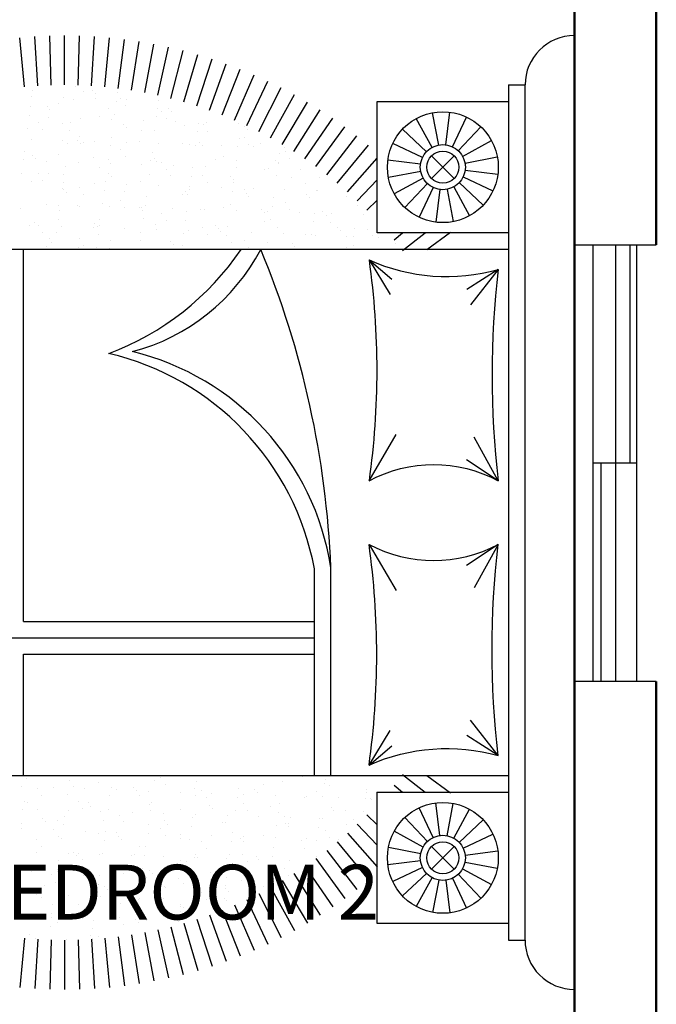
# Model space of a CAD drawing. Units: millimetres. Extents: x -857 to 54106, y -13666 to 13947.
# Tile 39 of 41: x 32096 to 33845, y 8428 to 11133. Entities that reach past the tile are written whole.
import ezdxf

# ---------------------------------------------------------------- set-up
doc = ezdxf.new("R2010")
doc.units = ezdxf.units.MM
for name, color, linetype, lineweight in [('A-ANNO-DIMS', 2, 'Continuous', 18), ('A-AREA-IDEN', 3, 'Continuous', 18), ('A-FURN', 21, 'Continuous', 18), ('A-GLAZ', 4, 'Continuous', 25), ('A-WALL', 7, 'Continuous', 50)]:
    doc.layers.add(name, color=color, linetype=linetype, lineweight=lineweight)
for name, color, linetype in [('A-FRN', 11, 'Continuous'), ('A-HT', 15, 'Continuous'), ('L-HT', 1, 'Continuous')]:
    doc.layers.add(name, color=color, linetype=linetype)
doc.styles.get("Standard").update_dxf_attribs({"font": 'arial.ttf'})
doc.dimstyles.new('ISO-25', dxfattribs={"dimtxt": 2.5, "dimasz": 2.5, "dimexe": 1.25, "dimexo": 0.625, "dimtad": 1, "dimtxsty": 'Standard', "dimcen": 2.5, "dimadec": 0, "dimazin": 0, "dimtfac": 1, "dimtmove": 0, "dimatfit": 3, "dimfxl": 1, "dimarcsym": 0})

# ---------------------------------------------------------------- blocks, each defined once
blk = doc.blocks.new('*X18')
at = {"color": 0}
for p, q in [((0.9679, 1.6809), (0.9679, 1.6809)), ((1.075, 1.6828), (1.075, 1.6828)), ((2.8341, 1.6809), (2.8341, 1.6809)), ((2.9037, 1.6769), (2.9037, 1.6769)), ((2.9444, 1.6822), (2.9444, 1.6822)), ((2.962, 1.6803), (2.962, 1.6803)), ((3.0971, 1.6852), (3.0971, 1.6852)), ((0.7154, 1.6491), (0.7154, 1.6491)), ((0.7341, 1.6496), (0.7341, 1.6496)), ((0.7667, 1.6544), (0.7667, 1.6544)), ((0.7927, 1.6578), (0.7927, 1.6578)), ((0.8333, 1.6632), (0.8333, 1.6632)), ((0.865, 1.6513), (0.865, 1.6513)), ((0.9013, 1.6721), (0.9013, 1.6721)), ((0.9155, 1.6474), (0.9155, 1.6474)), ((0.9273, 1.6756), (0.9273, 1.6756)), ((0.9929, 1.6507), (0.9929, 1.6507)), ((1.1279, 1.6556), (1.1279, 1.6556)), ((2.8098, 1.6645), (2.8098, 1.6645)), ((2.8777, 1.6734), (2.8777, 1.6734)), ((2.8812, 1.6623), (2.8812, 1.6623)), ((3.0813, 1.6605), (3.0813, 1.6605)), ((3.0905, 1.6521), (3.0905, 1.6521)), ((3.2843, 1.6561), (3.2843, 1.6561)), ((0.8149, 1.6302), (0.8149, 1.6302)), ((0.836, 1.6168), (0.836, 1.6168)), ((0.9247, 1.6389), (0.9247, 1.6389)), ((0.9706, 1.6305), (0.9706, 1.6305)), ((0.9917, 1.6171), (0.9917, 1.6171)), ((1.1185, 1.6429), (1.1185, 1.6429)), ((1.1263, 1.6308), (1.1263, 1.6308)), ((1.1474, 1.6173), (1.1474, 1.6173)), ((2.8391, 1.6339), (2.8391, 1.6339)), ((2.8602, 1.6205), (2.8602, 1.6205)), ((2.9017, 1.634), (2.9017, 1.634)), ((2.931, 1.6167), (2.931, 1.6167)), ((2.9948, 1.6342), (2.9948, 1.6342)), ((3.0159, 1.6207), (3.0159, 1.6207)), ((3.0326, 1.6357), (3.0326, 1.6357)), ((3.1505, 1.6345), (3.1505, 1.6345)), ((3.1605, 1.6351), (3.1605, 1.6351)), ((3.1716, 1.621), (3.1716, 1.621)), ((3.2956, 1.64), (3.2956, 1.64)), ((0.7652, 1.6035), (0.7652, 1.6035)), ((0.7744, 1.595), (0.7744, 1.595)), ((0.7976, 1.5996), (0.7976, 1.5996)), ((0.9326, 1.6044), (0.9326, 1.6044)), ((0.9682, 1.599), (0.9682, 1.599)), ((1.0635, 1.6061), (1.0635, 1.6061)), ((1.1683, 1.5973), (1.1683, 1.5973)), ((1.1775, 1.5889), (1.1775, 1.5889)), ((1.1914, 1.6055), (1.1914, 1.6055)), ((2.9402, 1.6082), (2.9402, 1.6082)), ((3.1002, 1.5888), (3.1002, 1.5888)), ((3.134, 1.6122), (3.134, 1.6122)), ((3.219, 1.5889), (3.219, 1.5889)), ((3.2311, 1.5905), (3.2311, 1.5905)), ((3.2596, 1.5943), (3.2596, 1.5943)), ((0.7562, 1.5681), (0.7562, 1.5681)), ((0.9119, 1.5684), (0.9119, 1.5684)), ((1.014, 1.5575), (1.014, 1.5575)), ((1.0676, 1.5687), (1.0676, 1.5687)), ((1.0819, 1.5665), (1.0819, 1.5665)), ((1.108, 1.5699), (1.108, 1.5699)), ((1.1311, 1.5592), (1.1311, 1.5592)), ((1.1486, 1.5753), (1.1486, 1.5753)), ((2.8373, 1.5846), (2.8373, 1.5846)), ((2.9361, 1.5721), (2.9361, 1.5721)), ((2.9652, 1.584), (2.9652, 1.584)), ((2.9837, 1.5683), (2.9837, 1.5683)), ((2.9905, 1.5588), (2.9905, 1.5588)), ((3.0584, 1.5678), (3.0584, 1.5678)), ((3.0844, 1.5712), (3.0844, 1.5712)), ((3.0918, 1.5724), (3.0918, 1.5724)), ((3.1251, 1.5765), (3.1251, 1.5765)), ((3.1838, 1.5666), (3.1838, 1.5666)), ((3.193, 1.5855), (3.193, 1.5855)), ((3.193, 1.5582), (3.193, 1.5582)), ((3.2475, 1.5727), (3.2475, 1.5727)), ((0.7373, 1.5533), (0.7373, 1.5533)), ((0.8128, 1.531), (0.8128, 1.531)), ((0.8179, 1.5552), (0.8179, 1.5552)), ((0.8388, 1.5345), (0.8388, 1.5345)), ((0.8681, 1.555), (0.8681, 1.555)), ((0.8794, 1.5398), (0.8794, 1.5398)), ((0.9474, 1.5488), (0.9474, 1.5488)), ((0.9734, 1.5522), (0.9734, 1.5522)), ((0.996, 1.5544), (0.996, 1.5544)), ((1.018, 1.5534), (1.018, 1.5534)), ((1.0272, 1.545), (1.0272, 1.545)), ((2.8152, 1.5357), (2.8152, 1.5357)), ((2.8559, 1.5411), (2.8559, 1.5411)), ((2.9049, 1.5377), (2.9049, 1.5377)), ((2.9238, 1.55), (2.9238, 1.55)), ((2.9498, 1.5535), (2.9498, 1.5535)), ((3.0358, 1.5394), (3.0358, 1.5394)), ((3.1637, 1.5388), (3.1637, 1.5388)), ((3.2987, 1.5436), (3.2987, 1.5436)), ((0.7042, 1.5167), (0.7042, 1.5167)), ((0.7448, 1.5221), (0.7448, 1.5221)), ((0.8007, 1.5032), (0.8007, 1.5032)), ((0.8553, 1.505), (0.8553, 1.505)), ((0.8677, 1.5096), (0.8677, 1.5096)), ((0.8769, 1.5011), (0.8769, 1.5011)), ((0.9358, 1.5081), (0.9358, 1.5081)), ((1.011, 1.5053), (1.011, 1.5053)), ((1.0666, 1.5098), (1.0666, 1.5098)), ((1.0707, 1.5051), (1.0707, 1.5051)), ((1.1667, 1.5056), (1.1667, 1.5056)), ((1.1945, 1.5091), (1.1945, 1.5091)), ((2.8334, 1.5245), (2.8334, 1.5245)), ((2.8795, 1.5087), (2.8795, 1.5087)), ((3.0334, 1.5227), (3.0334, 1.5227)), ((3.0352, 1.509), (3.0352, 1.509)), ((3.0427, 1.5143), (3.0427, 1.5143)), ((3.1909, 1.5093), (3.1909, 1.5093)), ((3.2365, 1.5183), (3.2365, 1.5183)), ((0.7207, 1.4913), (0.7207, 1.4913)), ((0.8764, 1.4916), (0.8764, 1.4916)), ((1.0321, 1.4919), (1.0321, 1.4919)), ((1.1878, 1.4921), (1.1878, 1.4921)), ((2.8404, 1.4882), (2.8404, 1.4882)), ((2.8831, 1.4789), (2.8831, 1.4789)), ((2.8924, 1.4704), (2.8924, 1.4704)), ((2.9006, 1.4953), (2.9006, 1.4953)), ((2.9683, 1.4876), (2.9683, 1.4876)), ((3.0563, 1.4955), (3.0563, 1.4955)), ((3.0862, 1.4744), (3.0862, 1.4744)), ((3.1034, 1.4925), (3.1034, 1.4925)), ((3.212, 1.4958), (3.212, 1.4958)), ((3.2343, 1.4942), (3.2343, 1.4942)), ((3.2862, 1.4727), (3.2862, 1.4727)), ((0.7174, 1.4657), (0.7174, 1.4657)), ((0.7266, 1.4572), (0.7266, 1.4572)), ((0.7404, 1.457), (0.7404, 1.457)), ((0.7966, 1.4429), (0.7966, 1.4429)), ((0.8713, 1.4586), (0.8713, 1.4586)), ((0.9204, 1.4613), (0.9204, 1.4613)), ((0.9523, 1.4432), (0.9523, 1.4432)), ((0.9992, 1.458), (0.9992, 1.458)), ((1.108, 1.4435), (1.108, 1.4435)), ((1.1205, 1.4595), (1.1205, 1.4595)), ((1.128, 1.4431), (1.128, 1.4431)), ((1.1297, 1.4511), (1.1297, 1.4511)), ((1.1342, 1.4629), (1.1342, 1.4629)), ((1.1541, 1.4465), (1.1541, 1.4465)), ((1.1947, 1.4519), (1.1947, 1.4519)), ((2.8208, 1.4466), (2.8208, 1.4466)), ((2.908, 1.4414), (2.908, 1.4414)), ((2.9765, 1.4469), (2.9765, 1.4469)), ((3.0389, 1.443), (3.0389, 1.443)), ((3.1045, 1.4444), (3.1045, 1.4444)), ((3.1305, 1.4478), (3.1305, 1.4478)), ((3.1322, 1.4472), (3.1322, 1.4472)), ((3.1668, 1.4424), (3.1668, 1.4424)), ((3.1712, 1.4532), (3.1712, 1.4532)), ((3.2391, 1.4621), (3.2391, 1.4621)), ((3.2651, 1.4655), (3.2651, 1.4655)), ((3.2879, 1.4475), (3.2879, 1.4475)), ((3.2954, 1.4643), (3.2954, 1.4643)), ((0.7701, 1.4174), (0.7701, 1.4174)), ((0.8589, 1.4076), (0.8589, 1.4076)), ((0.8849, 1.4111), (0.8849, 1.4111)), ((0.9255, 1.4164), (0.9255, 1.4164)), ((0.9389, 1.4118), (0.9389, 1.4118)), ((0.9701, 1.4157), (0.9701, 1.4157)), ((0.9794, 1.4072), (0.9794, 1.4072)), ((0.9935, 1.4254), (0.9935, 1.4254)), ((1.0195, 1.4288), (1.0195, 1.4288)), ((1.0601, 1.4341), (1.0601, 1.4341)), ((1.0698, 1.4134), (1.0698, 1.4134)), ((1.1732, 1.4112), (1.1732, 1.4112)), ((1.1977, 1.4128), (1.1977, 1.4128)), ((2.8353, 1.4089), (2.8353, 1.4089)), ((2.8613, 1.4124), (2.8613, 1.4124)), ((2.902, 1.4177), (2.902, 1.4177)), ((2.9359, 1.4306), (2.9359, 1.4306)), ((2.9699, 1.4267), (2.9699, 1.4267)), ((2.9959, 1.4301), (2.9959, 1.4301)), ((3.0366, 1.4354), (3.0366, 1.4354)), ((3.1359, 1.4288), (3.1359, 1.4288)), ((3.1451, 1.4204), (3.1451, 1.4204)), ((0.7243, 1.3899), (0.7243, 1.3899)), ((0.74, 1.3795), (0.74, 1.3795)), ((0.7503, 1.3934), (0.7503, 1.3934)), ((0.7909, 1.3987), (0.7909, 1.3987)), ((0.8039, 1.4069), (0.8039, 1.4069)), ((0.8957, 1.3798), (0.8957, 1.3798)), ((1.0514, 1.3801), (1.0514, 1.3801)), ((2.8436, 1.3919), (2.8436, 1.3919)), ((2.9199, 1.3835), (2.9199, 1.3835)), ((2.9715, 1.3913), (2.9715, 1.3913)), ((2.9856, 1.385), (2.9856, 1.385)), ((3.0756, 1.3838), (3.0756, 1.3838)), ((3.1065, 1.3961), (3.1065, 1.3961)), ((3.1886, 1.3805), (3.1886, 1.3805)), ((3.2313, 1.384), (3.2313, 1.384)), ((3.2374, 1.3978), (3.2374, 1.3978)), ((0.7436, 1.3606), (0.7436, 1.3606)), ((0.761, 1.3661), (0.761, 1.3661)), ((0.8198, 1.3718), (0.8198, 1.3718)), ((0.8291, 1.3633), (0.8291, 1.3633)), ((0.8744, 1.3623), (0.8744, 1.3623)), ((0.9168, 1.3664), (0.9168, 1.3664)), ((1.0023, 1.3617), (1.0023, 1.3617)), ((1.0229, 1.3673), (1.0229, 1.3673)), ((1.0725, 1.3667), (1.0725, 1.3667)), ((1.1374, 1.3665), (1.1374, 1.3665)), ((2.9409, 1.37), (2.9409, 1.37)), ((2.9948, 1.3765), (2.9948, 1.3765)), ((3.0967, 1.3703), (3.0967, 1.3703)), ((3.2524, 1.3706), (3.2524, 1.3706)), ((0.837, 1.3177), (0.837, 1.3177)), ((0.8726, 1.3235), (0.8726, 1.3235)), ((0.9927, 1.318), (0.9927, 1.318)), ((1.0726, 1.3217), (1.0726, 1.3217)), ((1.1484, 1.3183), (1.1484, 1.3183)), ((1.1741, 1.3197), (1.1741, 1.3197)), ((2.8353, 1.3411), (2.8353, 1.3411)), ((2.8445, 1.3326), (2.8445, 1.3326)), ((2.8611, 1.3214), (2.8611, 1.3214)), ((2.9112, 1.345), (2.9112, 1.345)), ((3.0169, 1.3217), (3.0169, 1.3217)), ((3.0383, 1.3367), (3.0383, 1.3367)), ((3.0421, 1.3467), (3.0421, 1.3467)), ((3.1506, 1.321), (3.1506, 1.321)), ((3.17, 1.3461), (3.17, 1.3461)), ((3.1726, 1.322), (3.1726, 1.322)), ((3.1766, 1.3244), (3.1766, 1.3244)), ((3.2173, 1.3298), (3.2173, 1.3298)), ((3.2384, 1.3349), (3.2384, 1.3349)), ((3.2476, 1.3265), (3.2476, 1.3265)), ((0.807, 1.3105), (0.807, 1.3105)), ((0.931, 1.2877), (0.931, 1.2877)), ((0.9421, 1.3154), (0.9421, 1.3154)), ((0.9716, 1.293), (0.9716, 1.293)), ((1.0396, 1.302), (1.0396, 1.302)), ((1.0656, 1.3054), (1.0656, 1.3054)), ((1.0729, 1.3171), (1.0729, 1.3171)), ((1.0818, 1.3133), (1.0818, 1.3133)), ((1.1062, 1.3108), (1.1062, 1.3108)), ((2.8467, 1.2956), (2.8467, 1.2956)), ((2.888, 1.2928), (2.888, 1.2928)), ((2.9074, 1.289), (2.9074, 1.289)), ((2.9481, 1.2943), (2.9481, 1.2943)), ((2.9746, 1.2949), (2.9746, 1.2949)), ((3.016, 1.3033), (3.016, 1.3033)), ((3.042, 1.3067), (3.042, 1.3067)), ((3.0827, 1.312), (3.0827, 1.312)), ((3.0881, 1.291), (3.0881, 1.291)), ((3.1097, 1.2998), (3.1097, 1.2998)), ((3.2406, 1.3015), (3.2406, 1.3015)), ((0.7467, 1.2643), (0.7467, 1.2643)), ((0.7704, 1.2665), (0.7704, 1.2665)), ((0.7964, 1.27), (0.7964, 1.27)), ((0.837, 1.2753), (0.837, 1.2753)), ((0.8776, 1.2659), (0.8776, 1.2659)), ((0.905, 1.2843), (0.905, 1.2843)), ((0.9223, 1.2779), (0.9223, 1.2779)), ((0.9315, 1.2694), (0.9315, 1.2694)), ((1.0055, 1.2653), (1.0055, 1.2653)), ((1.1253, 1.2734), (1.1253, 1.2734)), ((1.1405, 1.2702), (1.1405, 1.2702)), ((2.8045, 1.258), (2.8045, 1.258)), ((2.8135, 1.2766), (2.8135, 1.2766)), ((2.8814, 1.2855), (2.8814, 1.2855)), ((2.9602, 1.2583), (2.9602, 1.2583)), ((3.0973, 1.2826), (3.0973, 1.2826)), ((3.1159, 1.2586), (3.1159, 1.2586)), ((0.772, 1.234), (0.772, 1.234)), ((0.7803, 1.2543), (0.7803, 1.2543)), ((0.8014, 1.2409), (0.8014, 1.2409)), ((0.936, 1.2546), (0.936, 1.2546)), ((0.9571, 1.2412), (0.9571, 1.2412)), ((0.975, 1.2296), (0.975, 1.2296)), ((1.0918, 1.2549), (1.0918, 1.2549)), ((1.1128, 1.2414), (1.1128, 1.2414)), ((1.1751, 1.2278), (1.1751, 1.2278)), ((2.8256, 1.2446), (2.8256, 1.2446)), ((2.9143, 1.2487), (2.9143, 1.2487)), ((2.9378, 1.2472), (2.9378, 1.2472)), ((2.947, 1.2387), (2.947, 1.2387)), ((2.9813, 1.2448), (2.9813, 1.2448)), ((3.0452, 1.2503), (3.0452, 1.2503)), ((3.137, 1.2451), (3.137, 1.2451)), ((3.1408, 1.2427), (3.1408, 1.2427)), ((3.1731, 1.2497), (3.1731, 1.2497)), ((0.7812, 1.2255), (0.7812, 1.2255)), ((0.8102, 1.2142), (0.8102, 1.2142)), ((0.9452, 1.2191), (0.9452, 1.2191)), ((1.0761, 1.2207), (1.0761, 1.2207)), ((1.1843, 1.2194), (1.1843, 1.2194)), ((2.8499, 1.1992), (2.8499, 1.1992)), ((2.9778, 1.1986), (2.9778, 1.1986)), ((2.9905, 1.1989), (2.9905, 1.1989)), ((3.1128, 1.2035), (3.1128, 1.2035)), ((3.1967, 1.1976), (3.1967, 1.1976)), ((3.2227, 1.201), (3.2227, 1.201)), ((3.2437, 1.2051), (3.2437, 1.2051)), ((0.8247, 1.1857), (0.8247, 1.1857)), ((0.8773, 1.1925), (0.8773, 1.1925)), ((0.8807, 1.1696), (0.8807, 1.1696)), ((1.0086, 1.169), (1.0086, 1.169)), ((1.0177, 1.1696), (1.0177, 1.1696)), ((1.0248, 1.184), (1.0248, 1.184)), ((1.033, 1.1928), (1.033, 1.1928)), ((1.034, 1.1755), (1.034, 1.1755)), ((1.0857, 1.1786), (1.0857, 1.1786)), ((1.1117, 1.182), (1.1117, 1.182)), ((1.1437, 1.1739), (1.1437, 1.1739)), ((1.1523, 1.1874), (1.1523, 1.1874)), ((1.1887, 1.1931), (1.1887, 1.1931)), ((2.9015, 1.1962), (2.9015, 1.1962)), ((2.9942, 1.1709), (2.9942, 1.1709)), ((3.0572, 1.1965), (3.0572, 1.1965)), ((3.0621, 1.1799), (3.0621, 1.1799)), ((3.0881, 1.1833), (3.0881, 1.1833)), ((3.1288, 1.1887), (3.1288, 1.1887)), ((3.1906, 1.1971), (3.1906, 1.1971)), ((3.1998, 1.1887), (3.1998, 1.1887)), ((3.2129, 1.1968), (3.2129, 1.1968)), ((0.8165, 1.1432), (0.8165, 1.1432)), ((0.8425, 1.1466), (0.8425, 1.1466)), ((0.8745, 1.1401), (0.8745, 1.1401)), ((0.8831, 1.1519), (0.8831, 1.1519)), ((0.9511, 1.1609), (0.9511, 1.1609)), ((0.9771, 1.1643), (0.9771, 1.1643)), ((2.8189, 1.1479), (2.8189, 1.1479)), ((2.8402, 1.155), (2.8402, 1.155)), ((2.8596, 1.1532), (2.8596, 1.1532)), ((2.9175, 1.1523), (2.9175, 1.1523)), ((2.9275, 1.1622), (2.9275, 1.1622)), ((2.9535, 1.1656), (2.9535, 1.1656)), ((3.0403, 1.1533), (3.0403, 1.1533)), ((3.0484, 1.154), (3.0484, 1.154)), ((3.0495, 1.1448), (3.0495, 1.1448)), ((3.1763, 1.1534), (3.1763, 1.1534)), ((0.8133, 1.1179), (0.8133, 1.1179)), ((0.8207, 1.1291), (0.8207, 1.1291)), ((0.8418, 1.1157), (0.8418, 1.1157)), ((0.8837, 1.1316), (0.8837, 1.1316)), ((0.9484, 1.1227), (0.9484, 1.1227)), ((0.9764, 1.1294), (0.9764, 1.1294)), ((0.9975, 1.116), (0.9975, 1.116)), ((1.0775, 1.1356), (1.0775, 1.1356)), ((1.0792, 1.1244), (1.0792, 1.1244)), ((1.1321, 1.1297), (1.1321, 1.1297)), ((1.1532, 1.1162), (1.1532, 1.1162)), ((2.8449, 1.1328), (2.8449, 1.1328)), ((2.866, 1.1194), (2.866, 1.1194)), ((2.89, 1.1094), (2.89, 1.1094)), ((3.0006, 1.1331), (3.0006, 1.1331)), ((3.0217, 1.1196), (3.0217, 1.1196)), ((3.1563, 1.1334), (3.1563, 1.1334)), ((3.1774, 1.1199), (3.1774, 1.1199)), ((0.9272, 1.0918), (0.9272, 1.0918)), ((1.1273, 1.09), (1.1273, 1.09)), ((1.1365, 1.0816), (1.1365, 1.0816)), ((2.853, 1.1029), (2.853, 1.1029)), ((2.8992, 1.1009), (2.8992, 1.1009)), ((2.9809, 1.1023), (2.9809, 1.1023)), ((3.093, 1.105), (3.093, 1.105)), ((3.116, 1.1071), (3.116, 1.1071)), ((0.8839, 1.0733), (0.8839, 1.0733)), ((0.9177, 1.0673), (0.9177, 1.0673)), ((1.0118, 1.0727), (1.0118, 1.0727)), ((1.0734, 1.0676), (1.0734, 1.0676)), ((1.1318, 1.0552), (1.1318, 1.0552)), ((1.1468, 1.0775), (1.1468, 1.0775)), ((1.1578, 1.0586), (1.1578, 1.0586)), ((1.1984, 1.064), (1.1984, 1.064)), ((2.9206, 1.056), (2.9206, 1.056)), ((2.9419, 1.071), (2.9419, 1.071)), ((2.9427, 1.0611), (2.9427, 1.0611)), ((3.0515, 1.0577), (3.0515, 1.0577)), ((3.0976, 1.0713), (3.0976, 1.0713)), ((3.1082, 1.0565), (3.1082, 1.0565)), ((3.1342, 1.0599), (3.1342, 1.0599)), ((3.1428, 1.0594), (3.1428, 1.0594)), ((3.152, 1.0509), (3.152, 1.0509)), ((3.1749, 1.0653), (3.1749, 1.0653)), ((3.1794, 1.057), (3.1794, 1.057)), ((0.8165, 1.0215), (0.8165, 1.0215)), ((0.8626, 1.0198), (0.8626, 1.0198)), ((0.8886, 1.0232), (0.8886, 1.0232)), ((0.9292, 1.0285), (0.9292, 1.0285)), ((0.9515, 1.0264), (0.9515, 1.0264)), ((0.977, 1.0462), (0.977, 1.0462)), ((0.9862, 1.0377), (0.9862, 1.0377)), ((0.9972, 1.0375), (0.9972, 1.0375)), ((1.0232, 1.0409), (1.0232, 1.0409)), ((1.0638, 1.0463), (1.0638, 1.0463)), ((1.0824, 1.0281), (1.0824, 1.0281)), ((1.18, 1.0417), (1.18, 1.0417)), ((2.839, 1.0211), (2.839, 1.0211)), ((2.865, 1.0245), (2.865, 1.0245)), ((2.9057, 1.0298), (2.9057, 1.0298)), ((2.9736, 1.0388), (2.9736, 1.0388)), ((2.9996, 1.0422), (2.9996, 1.0422)), ((3.0403, 1.0475), (3.0403, 1.0475)), ((0.8267, 1.0023), (0.8267, 1.0023)), ((0.8359, 0.9938), (0.8359, 0.9938)), ((0.8611, 1.0039), (0.8611, 1.0039)), ((0.8822, 0.9905), (0.8822, 0.9905)), ((1.0168, 1.0042), (1.0168, 1.0042)), ((1.0297, 0.9979), (1.0297, 0.9979)), ((1.0379, 0.9908), (1.0379, 0.9908)), ((1.1725, 1.0045), (1.1725, 1.0045)), ((1.1936, 0.991), (1.1936, 0.991)), ((2.8562, 1.0065), (2.8562, 1.0065)), ((2.8853, 1.0076), (2.8853, 1.0076)), ((2.9064, 0.9942), (2.9064, 0.9942)), ((2.9841, 1.0059), (2.9841, 1.0059)), ((2.9925, 1.0155), (2.9925, 1.0155)), ((3.0017, 1.007), (3.0017, 1.007)), ((3.041, 1.0079), (3.041, 1.0079)), ((3.0621, 0.9944), (3.0621, 0.9944)), ((3.1191, 1.0108), (3.1191, 1.0108)), ((0.887, 0.9769), (0.887, 0.9769)), ((1.0149, 0.9763), (1.0149, 0.9763)), ((1.15, 0.9812), (1.15, 0.9812)), ((2.8421, 0.9716), (2.8421, 0.9716)), ((2.8514, 0.9631), (2.8514, 0.9631)), ((2.9238, 0.9597), (2.9238, 0.9597)), ((3.0452, 0.9672), (3.0452, 0.9672)), ((3.0547, 0.9613), (3.0547, 0.9613)), ((0.8794, 0.954), (0.8794, 0.954)), ((0.9546, 0.93), (0.9546, 0.93)), ((0.9581, 0.9421), (0.9581, 0.9421)), ((1.0795, 0.9523), (1.0795, 0.9523)), ((1.0855, 0.9317), (1.0855, 0.9317)), ((1.0887, 0.9438), (1.0887, 0.9438)), ((1.1138, 0.9424), (1.1138, 0.9424)), ((1.1779, 0.9318), (1.1779, 0.9318)), ((2.8266, 0.9455), (2.8266, 0.9455)), ((2.9823, 0.9458), (2.9823, 0.9458)), ((3.138, 0.9461), (3.138, 0.9461)), ((0.9292, 0.9084), (0.9292, 0.9084)), ((0.9347, 0.8998), (0.9347, 0.8998)), ((0.9384, 0.8999), (0.9384, 0.8999)), ((0.9753, 0.9052), (0.9753, 0.9052)), ((1.0433, 0.9141), (1.0433, 0.9141)), ((1.0693, 0.9175), (1.0693, 0.9175)), ((1.1099, 0.9229), (1.1099, 0.9229)), ((1.1322, 0.904), (1.1322, 0.904)), ((2.8593, 0.9102), (2.8593, 0.9102)), ((2.8949, 0.9233), (2.8949, 0.9233)), ((2.9111, 0.9011), (2.9111, 0.9011)), ((2.9518, 0.9064), (2.9518, 0.9064)), ((2.9872, 0.9096), (2.9872, 0.9096)), ((3.0197, 0.9154), (3.0197, 0.9154)), ((3.0457, 0.9188), (3.0457, 0.9188)), ((3.0864, 0.9242), (3.0864, 0.9242)), ((3.0949, 0.9216), (3.0949, 0.9216)), ((3.1041, 0.9131), (3.1041, 0.9131)), ((3.1223, 0.9144), (3.1223, 0.9144)), ((0.8902, 0.8806), (0.8902, 0.8806)), ((0.9015, 0.8787), (0.9015, 0.8787)), ((0.9087, 0.8964), (0.9087, 0.8964)), ((1.0181, 0.88), (1.0181, 0.88)), ((1.0572, 0.879), (1.0572, 0.879)), ((1.1531, 0.8848), (1.1531, 0.8848)), ((2.8172, 0.8887), (2.8172, 0.8887)), ((2.8851, 0.8977), (2.8851, 0.8977)), ((2.9257, 0.8824), (2.9257, 0.8824)), ((2.9446, 0.8777), (2.9446, 0.8777)), ((2.9468, 0.8689), (2.9468, 0.8689)), ((2.9538, 0.8692), (2.9538, 0.8692)), ((3.0814, 0.8827), (3.0814, 0.8827)), ((3.1025, 0.8692), (3.1025, 0.8692)), ((0.9226, 0.8653), (0.9226, 0.8653)), ((0.9819, 0.8601), (0.9819, 0.8601)), ((1.0783, 0.8655), (1.0783, 0.8655)), ((1.1819, 0.8583), (1.1819, 0.8583)), ((1.1912, 0.8499), (1.1912, 0.8499)), ((2.9269, 0.8633), (2.9269, 0.8633)), ((3.0578, 0.865), (3.0578, 0.865)), ((0.9578, 0.8337), (0.9578, 0.8337)), ((0.9985, 0.8169), (0.9985, 0.8169)), ((1.0316, 0.8145), (1.0316, 0.8145)), ((1.0887, 0.8354), (1.0887, 0.8354)), ((1.1542, 0.8172), (1.1542, 0.8172)), ((2.8035, 0.8253), (2.8035, 0.8253)), ((2.8625, 0.8138), (2.8625, 0.8138)), ((2.867, 0.8203), (2.867, 0.8203)), ((2.9904, 0.8132), (2.9904, 0.8132)), ((2.9973, 0.8294), (2.9973, 0.8294)), ((3.0227, 0.8206), (3.0227, 0.8206)), ((1.0212, 0.7836), (1.0212, 0.7836)), ((1.0214, 0.7818), (1.0214, 0.7818)), ((1.0409, 0.806), (1.0409, 0.806)), ((1.0894, 0.7907), (1.0894, 0.7907)), ((1.1154, 0.7941), (1.1154, 0.7941)), ((1.156, 0.7995), (1.156, 0.7995)), ((1.1563, 0.7885), (1.1563, 0.7885)), ((2.847, 0.7855), (2.847, 0.7855)), ((2.9979, 0.7831), (2.9979, 0.7831)), ((3.0471, 0.7838), (3.0471, 0.7838)), ((0.9808, 0.7764), (0.9808, 0.7764)), ((1.0844, 0.7662), (1.0844, 0.7662)), ((1.0976, 0.7538), (1.0976, 0.7538)), ((2.8104, 0.7569), (2.8104, 0.7569)), ((2.8227, 0.76), (2.8227, 0.76)), ((2.8633, 0.7653), (2.8633, 0.7653)), ((2.9301, 0.767), (2.9301, 0.767)), ((2.9312, 0.7743), (2.9312, 0.7743)), ((2.9572, 0.7777), (2.9572, 0.7777)), ((2.9661, 0.7572), (2.9661, 0.7572)), ((1.0918, 0.739), (1.0918, 0.739)), ((1.1187, 0.7403), (1.1187, 0.7403)), ((1.1341, 0.7206), (1.1341, 0.7206)), ((2.8314, 0.7435), (2.8314, 0.7435)), ((2.8968, 0.7399), (2.8968, 0.7399)), ((2.906, 0.7314), (2.906, 0.7314)), ((2.9871, 0.7437), (2.9871, 0.7437)), ((1.0389, 0.6917), (1.0389, 0.6917)), ((1.1433, 0.7121), (1.1433, 0.7121)), ((1.1594, 0.6922), (1.1594, 0.6922)), ((1.1946, 0.692), (1.1946, 0.692)), ((2.8656, 0.7175), (2.8656, 0.7175)), ((2.9073, 0.6951), (2.9073, 0.6951)), ((2.9495, 0.6916), (2.9495, 0.6916)), ((2.9935, 0.7169), (2.9935, 0.7169)), ((1.1355, 0.6673), (1.1355, 0.6673)), ((1.1615, 0.6707), (1.1615, 0.6707)), ((1.1868, 0.6723), (1.1868, 0.6723)), ((2.9332, 0.6706), (2.9332, 0.6706)), ((1.0675, 0.6584), (1.0675, 0.6584)), ((1.095, 0.6427), (1.095, 0.6427)), ((2.8427, 0.6332), (2.8427, 0.6332)), ((2.8507, 0.6317), (2.8507, 0.6317)), ((2.8688, 0.6366), (2.8688, 0.6366)), ((2.9094, 0.6419), (2.9094, 0.6419)), ((1.138, 0.6286), (1.138, 0.6286)), ((1.159, 0.6151), (1.159, 0.6151)), ((2.849, 0.6021), (2.849, 0.6021)), ((2.8688, 0.6212), (2.8688, 0.6212)), ((2.8718, 0.6183), (2.8718, 0.6183)), ((1.1626, 0.5958), (1.1626, 0.5958)), ((2.8013, 0.5694), (2.8013, 0.5694)), ((1.1816, 0.5439), (1.1816, 0.5439))]:
    blk.add_line(p, q, dxfattribs=at)
blk = doc.blocks.new('A$C6796526C')
at = {"layer": 'A-FRN'}
for p, q in [((0, 3), (2.9, 3)), ((2.75, 2.85), (0.15, 2.85)), ((0.15, 2.8), (0.15, 2.85)), ((2.75, 2.8), (2.75, 2.85)), ((0.15, 2.8), (2.75, 2.8)), ((0.2, 2.4), (0.2, 2.8)), ((0.6, 2.8), (0.6, 2.4)), ((2.3, 2.4), (2.3, 2.8)), ((2.7, 2.8), (2.7, 2.4)), ((0.6, 2.4), (0.2, 2.4)), ((2.7, 2.4), (2.3, 2.4))]:
    blk.add_line(p, q, dxfattribs=at)
blk.add_lwpolyline([(0.65, 2.8), (0.65, 0.9), (2.25, 0.9), (2.25, 2.8)], dxfattribs=at)
for points in [[(0.6821, 2.3755, 0.175461), (0.7109, 2.7686)], [(0.7109, 2.7686, 0.059544), (1.3533, 2.7686)], [(1.3533, 2.3755, -0.248743), (1.3533, 2.7686)], [(2.1891, 2.7686, -0.059544), (1.5467, 2.7686)], [(1.5467, 2.3755, 0.248743), (1.5467, 2.7686)], [(2.2179, 2.3755, -0.175461), (2.1891, 2.7686)], [(0.6821, 2.3755, -0.069628), (1.3533, 2.3755)], [(2.2179, 2.3755, 0.069628), (1.5467, 2.3755)], [(2.25, 2.2594), (1.6173, 2.2594, 0.303651), (0.9607, 1.6568, 0.210515), (0.65, 2.0462)]]:
    blk.add_lwpolyline(points, format="xyb", dxfattribs=at)
for centre, radius in [((0.4, 2.6), 0.1686), ((2.5, 2.6), 0.1686), ((0.4, 2.6), 0.0686), ((2.5, 2.6), 0.0686)]:
    blk.add_circle(centre, radius, dxfattribs=at)
for centre, radius, start, end in [((0.15, 3), 0.15, 180, 270), ((2.75, 3), 0.15, 270, 0), ((1.7313, -0.5592), 2.8209, 92.3174, 112.5397)]:
    blk.add_arc(centre, radius, start, end, dxfattribs=at)
at = {"layer": 'A-HT'}
for p, q in [((0.65, 2.5511), (0.5977, 2.6231)), ((2.25, 2.5511), (2.3023, 2.6231)), ((0.6532, 2.4772), (0.6, 2.5458)), ((2.2468, 2.4772), (2.3, 2.5458)), ((0.6213, 2.4517), (0.6, 2.4775)), ((2.2787, 2.4517), (2.3, 2.4775)), ((0.4749, 2.3097), (0.3724, 2.4)), ((0.5023, 2.3399), (0.4384, 2.4)), ((0.5308, 2.3692), (0.5, 2.4)), ((2.3692, 2.3692), (2.4, 2.4)), ((2.3977, 2.3399), (2.4616, 2.4)), ((2.4251, 2.3097), (2.5276, 2.4)), ((0.4483, 2.2787), (0.3328, 2.3743)), ((2.4517, 2.2787), (2.5672, 2.3743)), ((0.4228, 2.2468), (0.3043, 2.3387)), ((2.4772, 2.2468), (2.5957, 2.3387)), ((0.3983, 2.2141), (0.2769, 2.3023)), ((2.5017, 2.2141), (2.6231, 2.3023)), ((0.3748, 2.1807), (0.2507, 2.265)), ((2.5252, 2.1807), (2.6493, 2.265)), ((0.3524, 2.1466), (0.2257, 2.2269)), ((2.5476, 2.1466), (2.6743, 2.2269)), ((0.331, 2.1118), (0.2019, 2.1881)), ((2.569, 2.1118), (2.6981, 2.1881)), ((0.3108, 2.0763), (0.1794, 2.1485)), ((2.5892, 2.0763), (2.7206, 2.1485)), ((0.2917, 2.0402), (0.158, 2.1083)), ((2.6083, 2.0402), (2.742, 2.1083)), ((0.2737, 2.0035), (0.138, 2.0674)), ((2.6263, 2.0035), (2.762, 2.0674)), ((0.2569, 1.9663), (0.1193, 2.0259)), ((2.6431, 1.9663), (2.7807, 2.0259)), ((0.2413, 1.9286), (0.1018, 1.9838)), ((2.6587, 1.9286), (2.7982, 1.9838)), ((0.2269, 1.8904), (0.0857, 1.9412)), ((2.6731, 1.8904), (2.8143, 1.9412)), ((0.2136, 1.8517), (0.071, 1.8981)), ((2.6864, 1.8517), (2.829, 1.8981)), ((0.2016, 1.8127), (0.0576, 1.8545)), ((2.6984, 1.8127), (2.8424, 1.8545)), ((0.1908, 1.7733), (0.0456, 1.8106)), ((2.7092, 1.7733), (2.8544, 1.8106)), ((0.1813, 1.7336), (0.0349, 1.7663)), ((2.7187, 1.7336), (2.8651, 1.7663)), ((0.173, 1.6936), (0.0257, 1.7217)), ((2.727, 1.6936), (2.8743, 1.7217)), ((0.166, 1.6534), (0.0179, 1.6768)), ((2.734, 1.6534), (2.8821, 1.6768)), ((0.1603, 1.6129), (0.0114, 1.6317)), ((2.7397, 1.6129), (2.8886, 1.6317)), ((0.1558, 1.5723), (0.0064, 1.5865)), ((2.7442, 1.5723), (2.8936, 1.5865)), ((0.1526, 1.5316), (0.0029, 1.541)), ((2.7474, 1.5316), (2.8971, 1.541)), ((0.1506, 1.4908), (0.0007, 1.4955)), ((2.7494, 1.4908), (2.8993, 1.4955)), ((0.15, 1.45), (0, 1.45)), ((2.75, 1.45), (2.9, 1.45)), ((0.1506, 1.4092), (0.0007, 1.4045)), ((2.7494, 1.4092), (2.8993, 1.4045)), ((0.1526, 1.3684), (0.0029, 1.359)), ((2.7474, 1.3684), (2.8971, 1.359)), ((0.1558, 1.3277), (0.0064, 1.3135)), ((2.7442, 1.3277), (2.8936, 1.3135))]:
    blk.add_line(p, q, dxfattribs=at)
at = {"layer": 'L-HT'}
for p, q in [((0.3873, 2.6674), (0.3687, 2.7656)), ((0.4087, 2.668), (0.4214, 2.7672)), ((0.7109, 2.7686), (0.8188, 2.6839)), ((0.7109, 2.7686), (0.7717, 2.6727)), ((1.3533, 2.7686), (1.2212, 2.6952)), ((1.3533, 2.7686), (1.2893, 2.6715)), ((1.5467, 2.7686), (1.6107, 2.6715)), ((1.5467, 2.7686), (1.6788, 2.6952)), ((2.1891, 2.7686), (2.0812, 2.6839)), ((2.1891, 2.7686), (2.1283, 2.6727)), ((2.4913, 2.668), (2.4786, 2.7672)), ((2.5127, 2.6674), (2.5313, 2.7656)), ((0.3671, 2.6601), (0.319, 2.7478)), ((0.4293, 2.662), (0.472, 2.7524)), ((2.4707, 2.662), (2.428, 2.7524)), ((2.5329, 2.6601), (2.581, 2.7478)), ((0.3501, 2.647), (0.2773, 2.7156)), ((0.447, 2.6499), (0.5156, 2.7227)), ((2.453, 2.6499), (2.3844, 2.7227)), ((2.5499, 2.647), (2.6227, 2.7156)), ((0.338, 2.6293), (0.2476, 2.672)), ((0.4601, 2.6329), (0.5478, 2.681)), ((2.4399, 2.6329), (2.3522, 2.681)), ((2.562, 2.6293), (2.6524, 2.672)), ((0.332, 2.6087), (0.2328, 2.6214)), ((0.3657, 2.5657), (0.4343, 2.6343)), ((0.4343, 2.5657), (0.3657, 2.6343)), ((0.4674, 2.6127), (0.5656, 2.6313)), ((2.4326, 2.6127), (2.3344, 2.6313)), ((2.4657, 2.5657), (2.5343, 2.6343)), ((2.5343, 2.5657), (2.4657, 2.6343)), ((2.568, 2.6087), (2.6672, 2.6214)), ((0.3326, 2.5873), (0.2344, 2.5687)), ((0.468, 2.5913), (0.5672, 2.5786)), ((2.432, 2.5913), (2.3328, 2.5786)), ((2.5674, 2.5873), (2.6656, 2.5687)), ((0.3399, 2.5671), (0.2522, 2.519)), ((0.353, 2.5501), (0.2844, 2.4773)), ((0.4499, 2.553), (0.5227, 2.4844)), ((0.462, 2.5707), (0.5524, 2.528)), ((2.438, 2.5707), (2.3476, 2.528)), ((2.4501, 2.553), (2.3773, 2.4844)), ((2.547, 2.5501), (2.6156, 2.4773)), ((2.5601, 2.5671), (2.6478, 2.519)), ((0.3707, 2.538), (0.328, 2.4476)), ((0.3913, 2.532), (0.3786, 2.4328)), ((0.4127, 2.5326), (0.4313, 2.4344)), ((0.4329, 2.5399), (0.481, 2.4522)), ((2.4671, 2.5399), (2.419, 2.4522)), ((2.4873, 2.5326), (2.4687, 2.4344)), ((2.5087, 2.532), (2.5214, 2.4328)), ((2.5293, 2.538), (2.572, 2.4476)), ((1.3533, 2.3755), (1.2125, 2.4585)), ((1.5467, 2.3755), (1.6875, 2.4585)), ((0.6821, 2.3755), (0.7405, 2.4447)), ((0.6821, 2.3755), (0.7872, 2.4395)), ((2.2179, 2.3755), (2.1128, 2.4395)), ((2.2179, 2.3755), (2.1595, 2.4447)), ((2.25, 2.2094), (1.6212, 2.2094)), ((1.7809, 1.3249), (1.7809, 2.2094)), ((1.8309, 0.9), (1.8309, 2.2094)), ((1.8809, 1.3249), (1.8809, 2.2094)), ((1.7809, 1.3249), (0.65, 1.3249)), ((2.25, 1.3249), (1.8809, 1.3249))]:
    blk.add_line(p, q, dxfattribs=at)
for centre in [(0.4, 2.6), (2.5, 2.6)]:
    blk.add_circle(centre, 0.0486, dxfattribs=at)
for centre, radius, start, end in [((1.7721, 1.396), 0.8272, 100.5107, 166.872), ((0.1786, 1.2908), 0.8406, 20.4105, 55.8901)]:
    blk.add_arc(centre, radius, start, end, dxfattribs=at)
at = {"layer": 'A-HT', "extrusion": (0, 0, -1), "zscale": -1, "rotation": 180}
blk.add_blockref('*X18', (0.55, 3), dxfattribs=at)
blk = doc.blocks.new('WIN-1200')
for p, q in [((9371.3, 11750.2), (10571.3, 11750.2)), ((9971.3, 11750.2), (9971.3, 11630.7)), ((9371.3, 11731.7), (9971.3, 11731.7)), ((9371.3, 11691.7), (10571.3, 11691.7)), ((9971.3, 11651.7), (10571.3, 11651.7)), ((10571.3, 11630.7), (9371.3, 11630.7))]:
    blk.add_line(p, q)
for points in [[(9371.3, 11579.2), (9371.3, 11804.2)], [(10571.3, 11804.2), (10571.3, 11579.2)]]:
    blk.add_lwpolyline(points)
blk = doc.blocks.new('*D47')
at = {"layer": 'A-ANNO-DIMS', "color": 0, "lineweight": -2, "transparency": 16777216}
for p, q in [((30909.3, 8468.4), (30909.3, 8061.1)), ((33620.1, 8468.4), (33620.1, 8061.1)), ((30911.8, 8062.4), (33617.6, 8062.4))]:
    blk.add_line(p, q, dxfattribs=at)
at = {"layer": 'A-ANNO-DIMS', "color": 0, "transparency": 16777216}
for points in [[(30911.8, 8062.8), (30911.8, 8062), (30909.3, 8062.4)], [(33617.6, 8062.8), (33617.6, 8062), (33620.1, 8062.4)]]:
    blk.add_solid(points, dxfattribs=at)
at = {"layer": 'Defpoints', "color": 0, "transparency": 16777216}
for p in [(30909.3, 8469), (33620.1, 8469), (33620.1, 8062.4)]:
    blk.add_point(p, dxfattribs=at)
at = {"layer": 'A-ANNO-DIMS', "color": 0, "transparency": 16777216, "insert": (32264.7, 8064.3), "char_height": 2.5, "attachment_point": 5}
blk.add_mtext('ROUND BED 2711 TYP.', dxfattribs=at)

msp = doc.modelspace()

# ---------------------------------------------------------------- linework, layer by layer
at = {"layer": 'A-WALL'}
for p, q in [((33845.08, 11629.231), (33845.08, 10514.82)), ((33620.079, 11404.231), (33620.079, 8154.231)), ((33845.069, 9314.82), (33845.063, 8154.231))]:
    msp.add_line(p, q, dxfattribs=at)

# ---------------------------------------------------------------- block references
at = {"layer": 'A-FURN', "xscale": 903.6084929786902, "yscale": 903.6084929786902, "zscale": 903.6084929786902, "rotation": 269.9999999999988}
msp.add_blockref('A$C6796526C', (30909.253, 11089.463), dxfattribs=at)
at = {"layer": 'A-GLAZ', "rotation": 270.0000000000007}
msp.add_blockref('WIN-1200', (22040.838, 19886.161), dxfattribs=at)

# ---------------------------------------------------------------- texts
at = {"layer": 'A-AREA-IDEN', "insert": (31924.893, 8811.521), "char_height": 150.48461, "attachment_point": 1}
msp.add_mtext_dynamic_manual_height_columns('\\pxt0;BEDROOM 2', width=2554.22693, gutter_width=18810.576, heights=[2595.835], dxfattribs=at)

# ---------------------------------------------------------------- dimensions: what is measured, and where the dimension line sits
at = {"layer": 'A-ANNO-DIMS'}
dim = msp.add_linear_dim(base=(33620.079, 8062.375), p1=(30909.254, 8468.999), p2=(33620.079, 8468.999), text='ROUND BED <> TYP.', dimstyle='ISO-25', override={"dimdec": 0, "dimrnd": 0, "dimzin": 0, "dimlunit": 2}, dxfattribs=at)
dim.commit()
dim.dimension.update_dxf_attribs({"geometry": '*D47', "text_midpoint": (32264.666, 8064.293)})

doc.saveas('drawing.dxf')
